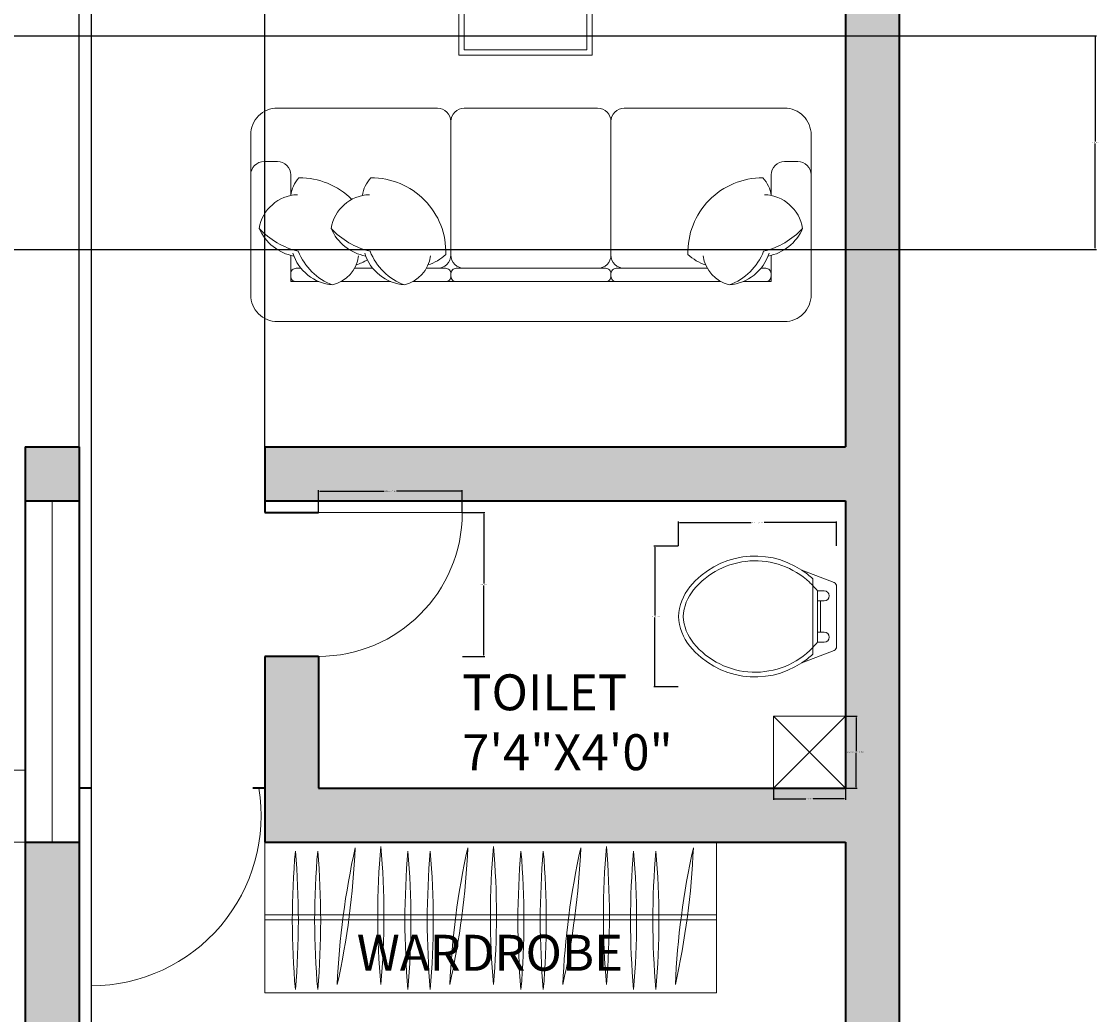
# Model space of a CAD drawing. Units: inches. Extents: x 37 to 706, y -568 to 110.
# Tile 17 of 24: x 526 to 706, y -398 to -233. Entities that reach past the tile are written whole.
import ezdxf

# ---------------------------------------------------------------- set-up
doc = ezdxf.new("R2010")
doc.units = ezdxf.units.IN
doc.header["$MEASUREMENT"] = 0
for name, color, linetype, lineweight in [('A-ANNO-DIMS', 2, 'Continuous', 18), ('A-ANNO-TEXT', 7, 'Continuous', 18), ('A-AREA-IDEN', 7, 'Continuous', 18), ('A-DOOR', 4, 'Continuous', 18), ('A-FLOR-CASE', 9, 'Continuous', 18), ('A-FLOR-FIXT', 9, 'Continuous', 18), ('A-FLOR-OPEN', 8, 'Continuous', 13), ('A-FLOR-STRS', 7, 'Continuous', 18), ('A-FURN', 8, 'Continuous', 13), ('A-GLAZ', 4, 'Continuous', 18), ('A-WALL', 7, 'Continuous', 35), ('A-WALL-PATT', 252, 'Continuous', 13)]:
    doc.layers.add(name, color=color, linetype=linetype, lineweight=lineweight)
doc.styles.get("Standard").update_dxf_attribs({"font": 'arial.ttf'})
doc.dimstyles.get("Standard").update_dxf_attribs({"dimtxt": 0.18, "dimasz": 0.18, "dimexe": 0.18, "dimexo": 0.0625, "dimgap": 0.09, "dimtad": 0, "dimtih": 1, "dimtoh": 1, "dimdec": 0, "dimzin": 0, "dimdsep": 46, "dimlunit": 3, "dimtxsty": 'Standard', "dimcen": 0.09, "dimadec": 0, "dimazin": 0, "dimtfac": 1, "dimtdec": 0, "dimtofl": 0, "dimtmove": 0, "dimatfit": 3, "dimfxl": 1, "dimtolj": 1, "dimtzin": 0, "dimarcsym": 0})

# ---------------------------------------------------------------- blocks, each defined once
blk = doc.blocks.new('WARDROBE-DOUBLE')
for p, q in [((75.49, 25.16), (0, 25.16)), ((0, 25.16), (0, 0)), ((75.49, 25.16), (75.49, 0)), ((75.49, 13), (0, 13)), ((75.49, 12.16), (0, 12.16)), ((75.49, 0), (0, 0))]:
    blk.add_line(p, q)
for centre, start, end in [((137.01, 12.08), 175.0028, 184.9972), ((-126.78, 12.08), 355.0028, 4.9972), ((140.74, 12.08), 175.0028, 184.9972), ((-123.05, 12.08), 355.0028, 4.9972), ((-117.16, 29.99), 347.508, 357.5023), ((144.38, -4.42), 167.508, 177.5023), ((151.29, 12.89), 175.0028, 184.9972), ((-112.5, 12.89), 355.0028, 4.9972), ((155.82, 12.08), 175.0028, 184.9972), ((-107.97, 12.08), 355.0028, 4.9972), ((159.55, 12.08), 175.0028, 184.9972), ((-104.24, 12.08), 355.0028, 4.9972), ((-98.35, 29.99), 347.508, 357.5023), ((163.19, -4.42), 167.508, 177.5023), ((170.1, 12.89), 175.0028, 184.9972), ((-93.69, 12.89), 355.0028, 4.9972), ((174.7, 12.08), 175.0028, 184.9972), ((-89.09, 12.08), 355.0028, 4.9972), ((178.43, 12.08), 175.0028, 184.9972), ((-85.36, 12.08), 355.0028, 4.9972), ((182.06, -4.42), 167.508, 177.5023), ((-79.47, 29.99), 347.508, 357.5023), ((188.97, 12.89), 175.0028, 184.9972), ((-74.82, 12.89), 355.0028, 4.9972), ((193.51, 12.08), 175.0028, 184.9972), ((-70.28, 12.08), 355.0028, 4.9972), ((197.24, 12.08), 175.0028, 184.9972), ((-66.55, 12.08), 355.0028, 4.9972), ((200.87, -4.42), 167.508, 177.5023), ((-60.66, 29.99), 347.508, 357.5023)]:
    blk.add_arc(centre, 132.4, start, end)
blk = doc.blocks.new('WC-PLAN')
for p, q in [((22.41, 16.39), (22.41, 15.28)), ((22.41, 15.28), (22.41, 10.09)), ((22.41, 4.89), (22.41, 10.09)), ((22.41, 4.89), (22.41, 3.79))]:
    blk.add_line(p, q)
for points in [[(20.6, 17.82, 0.383919), (1.9, 15.05, 0.163732), (0, 10.09, 0.359733)], [(21.87, 15.81, 0.431639), (2.51, 14.55, 0.162618), (0.79, 10.09, 0.470877)], [(22.41, 16.39, 0.040937), (20.6, 17.82, 0.163732)], [(26.41, 10.09), (26.41, 15.13, 0.31031), (25.98, 15.75), (20.6, 17.82, 0.209071)], [(22.41, 15.28, 0.014165), (21.87, 15.81, 0.162618)], [(23.21, 14.37, 0.022712), (22.41, 15.28, 0.162618)], [(23.21, 10.09), (23.21, 14.37, 0.022712)], [(23.21, 14.37), (24.32, 14.37, -1), (24.32, 12.69), (23.74, 12.69)], [(20.6, 2.36, -0.383919), (1.9, 5.12, -0.163732), (0, 10.09, -0.359733)], [(22.41, 4.89, -0.448546), (2.51, 5.63, -0.162618), (0.79, 10.09, -0.470877)], [(26.41, 10.09), (26.41, 5.05, -0.31031), (25.98, 4.43), (20.6, 2.36, -0.209071)], [(23.21, 10.09), (23.21, 5.8, -0.476108)], [(23.21, 5.8), (24.32, 5.8, 1), (24.32, 7.49), (23.74, 7.49)], [(23.21, 5.8, -0.022712), (22.41, 4.89, -0.162618)], [(22.41, 3.79, -0.040937), (20.6, 2.36, -0.163732)]]:
    blk.add_lwpolyline(points, format="xyb")
for points in [[(23.74, 12.69), (23.21, 12.69)], [(23.74, 7.49), (23.74, 12.69)], [(23.74, 7.49), (23.21, 7.49)]]:
    blk.add_lwpolyline(points)
blk = doc.blocks.new('COFFEE-TABLE-SQUARE')
at = {"ltscale": 0.03}
blk.add_lwpolyline([(22.29, 0), (0, 0), (0, 22.29), (22.29, 22.29)], close=True, dxfattribs=at)
blk.add_lwpolyline([(0.89, 0.89), (21.4, 0.89), (21.4, 21.4), (0.89, 21.4)], close=True)
blk = doc.blocks.new('DOOR-SWING-24')
blk.add_line((0, 0), (0, 24))
blk.add_arc((0, 0), 24, 0, 90)
blk = doc.blocks.new('FLOOR-OPENING-12-SQ')
for p, q in [((0, 0), (0, 12)), ((0, 12), (12, 12)), ((12, 12), (0, 0)), ((12, 0), (0, 12))]:
    blk.add_line(p, q)
blk = doc.blocks.new('*D17')
at = {"layer": 'A-ANNO-DIMS', "color": 0, "lineweight": -2, "transparency": 16777216}
for p, q in [((575.96, -314.65), (575.96, -310.93)), ((576.14, -311.11), (586.91, -311.11)), ((599.78, -311.11), (589, -311.11)), ((599.96, -314.65), (599.96, -310.93))]:
    blk.add_line(p, q, dxfattribs=at)
at = {"layer": 'A-ANNO-DIMS', "color": 0, "transparency": 16777216}
for points in [[(576.14, -311.08), (576.14, -311.14), (575.96, -311.11)], [(599.78, -311.08), (599.78, -311.14), (599.96, -311.11)]]:
    blk.add_solid(points, dxfattribs=at)
at = {"layer": 'Defpoints', "color": 0, "transparency": 16777216}
for p in [(599.96, -311.11), (575.96, -314.71), (599.96, -314.71)]:
    blk.add_point(p, dxfattribs=at)
at = {"layer": 'A-ANNO-DIMS', "color": 0, "transparency": 16777216, "insert": (587.96, -311.11), "char_height": 0.18, "attachment_point": 5}
blk.add_mtext('\\A1;DOOR 2\'-0" TYP.', dxfattribs=at)
blk = doc.blocks.new('*D18')
at = {"layer": 'A-ANNO-DIMS', "color": 0, "lineweight": -2, "transparency": 16777216}
for p, q in [((600.02, -314.71), (603.74, -314.71)), ((603.56, -314.89), (603.56, -326.53)), ((603.56, -338.53), (603.56, -326.89)), ((600.02, -338.71), (603.74, -338.71))]:
    blk.add_line(p, q, dxfattribs=at)
at = {"layer": 'A-ANNO-DIMS', "color": 0, "transparency": 16777216}
for points in [[(603.53, -314.89), (603.59, -314.89), (603.56, -314.71)], [(603.53, -338.53), (603.59, -338.53), (603.56, -338.71)]]:
    blk.add_solid(points, dxfattribs=at)
at = {"layer": 'Defpoints', "color": 0, "transparency": 16777216}
for p in [(599.96, -314.71), (599.96, -338.71), (603.56, -338.71)]:
    blk.add_point(p, dxfattribs=at)
at = {"layer": 'A-ANNO-DIMS', "color": 0, "transparency": 16777216, "insert": (603.56, -326.71), "char_height": 0.18, "attachment_point": 5}
blk.add_mtext('\\A1;2\'-0" TYP.', dxfattribs=at)
blk = doc.blocks.new('*D25')
at = {"layer": 'A-ANNO-DIMS', "color": 0, "lineweight": -2, "transparency": 16777216}
for p, q in [((636.09, -320.26), (636.09, -316.18)), ((636.27, -316.36), (648.2, -316.36)), ((662.32, -316.36), (650.39, -316.36)), ((662.5, -320.26), (662.5, -316.18))]:
    blk.add_line(p, q, dxfattribs=at)
at = {"layer": 'A-ANNO-DIMS', "color": 0, "transparency": 16777216}
for points in [[(636.27, -316.33), (636.27, -316.39), (636.09, -316.36)], [(662.32, -316.33), (662.32, -316.39), (662.5, -316.36)]]:
    blk.add_solid(points, dxfattribs=at)
at = {"layer": 'Defpoints', "color": 0, "transparency": 16777216}
for p in [(662.5, -316.36), (636.09, -320.32), (662.5, -320.32)]:
    blk.add_point(p, dxfattribs=at)
at = {"layer": 'A-ANNO-DIMS', "color": 0, "transparency": 16777216, "insert": (649.3, -316.36), "char_height": 0.18, "attachment_point": 5}
blk.add_mtext('\\A1;WC 2\'-2 1/2" TYP.', dxfattribs=at)
blk = doc.blocks.new('*D26')
at = {"layer": 'A-ANNO-DIMS', "color": 0, "lineweight": -2, "transparency": 16777216}
for p, q in [((636.03, -320.32), (631.95, -320.32)), ((632.13, -320.5), (632.13, -331.87)), ((632.13, -343.61), (632.13, -332.24)), ((636.03, -343.79), (631.95, -343.79))]:
    blk.add_line(p, q, dxfattribs=at)
at = {"layer": 'A-ANNO-DIMS', "color": 0, "transparency": 16777216}
for points in [[(632.1, -320.5), (632.16, -320.5), (632.13, -320.32)], [(632.1, -343.61), (632.16, -343.61), (632.13, -343.79)]]:
    blk.add_solid(points, dxfattribs=at)
at = {"layer": 'Defpoints', "color": 0, "transparency": 16777216}
for p in [(632.13, -320.32), (636.09, -320.32), (636.09, -343.79)]:
    blk.add_point(p, dxfattribs=at)
at = {"layer": 'A-ANNO-DIMS', "color": 0, "transparency": 16777216, "insert": (632.13, -332.05), "char_height": 0.18, "attachment_point": 5}
blk.add_mtext('\\A1;1\'-11 1/2" TYP.', dxfattribs=at)
blk = doc.blocks.new('*D37')
at = {"layer": 'A-ANNO-DIMS', "color": 0, "lineweight": -2, "transparency": 16777216}
for p, q in [((664.02, -348.71), (665.94, -348.71)), ((665.76, -348.89), (665.76, -354.53)), ((665.76, -360.53), (665.76, -354.89)), ((664.02, -360.71), (665.94, -360.71))]:
    blk.add_line(p, q, dxfattribs=at)
at = {"layer": 'A-ANNO-DIMS', "color": 0, "transparency": 16777216}
for points in [[(665.73, -348.89), (665.79, -348.89), (665.76, -348.71)], [(665.73, -360.53), (665.79, -360.53), (665.76, -360.71)]]:
    blk.add_solid(points, dxfattribs=at)
at = {"layer": 'Defpoints', "color": 0, "transparency": 16777216}
for p in [(663.96, -348.71), (665.76, -348.71), (663.96, -360.71)]:
    blk.add_point(p, dxfattribs=at)
at = {"layer": 'A-ANNO-DIMS', "color": 0, "transparency": 16777216, "insert": (665.76, -354.71), "char_height": 0.18, "attachment_point": 5}
blk.add_mtext('\\A1;FLOOR OPENING 1\'-0" TYP.', dxfattribs=at)
blk = doc.blocks.new('*D38')
at = {"layer": 'A-ANNO-DIMS', "color": 0, "lineweight": -2, "transparency": 16777216}
for p, q in [((651.96, -360.77), (651.96, -362.69)), ((663.96, -360.77), (663.96, -362.69)), ((652.14, -362.51), (657.33, -362.51)), ((663.78, -362.51), (658.59, -362.51))]:
    blk.add_line(p, q, dxfattribs=at)
at = {"layer": 'A-ANNO-DIMS', "color": 0, "transparency": 16777216}
for points in [[(652.14, -362.48), (652.14, -362.54), (651.96, -362.51)], [(663.78, -362.48), (663.78, -362.54), (663.96, -362.51)]]:
    blk.add_solid(points, dxfattribs=at)
at = {"layer": 'Defpoints', "color": 0, "transparency": 16777216}
for p in [(651.96, -360.71), (663.96, -360.71), (663.96, -362.51)]:
    blk.add_point(p, dxfattribs=at)
at = {"layer": 'A-ANNO-DIMS', "color": 0, "transparency": 16777216, "insert": (657.96, -362.51), "char_height": 0.18, "attachment_point": 5}
blk.add_mtext('\\A1;1\'-0" TYP.', dxfattribs=at)
blk = doc.blocks.new('*D50')
at = {"layer": 'A-ANNO-DIMS', "color": 0, "lineweight": -2, "transparency": 16777216}
for p, q in [((340.88, -235.09), (705.89, -235.09)), ((705.71, -235.27), (705.71, -252.74)), ((705.71, -270.57), (705.71, -253.1)), ((340.88, -270.75), (705.89, -270.75))]:
    blk.add_line(p, q, dxfattribs=at)
at = {"layer": 'A-ANNO-DIMS', "color": 0, "transparency": 16777216}
for points in [[(705.68, -235.27), (705.74, -235.27), (705.71, -235.09)], [(705.68, -270.57), (705.74, -270.57), (705.71, -270.75)]]:
    blk.add_solid(points, dxfattribs=at)
at = {"layer": 'Defpoints', "color": 0, "transparency": 16777216}
for p in [(340.81, -235.09), (340.81, -270.75), (705.71, -270.75)]:
    blk.add_point(p, dxfattribs=at)
at = {"layer": 'A-ANNO-DIMS', "color": 0, "transparency": 16777216, "insert": (705.71, -252.92), "char_height": 0.18, "attachment_point": 5}
blk.add_mtext('\\A1;2\'-11 1/2"', dxfattribs=at)
blk = doc.blocks.new('*D52')
at = {"layer": 'A-ANNO-DIMS', "color": 0, "lineweight": -2, "transparency": 16777216}
for p, q in [((535.96, -303.65), (535.96, 84.22)), ((536.14, 84.04), (551.13, 84.04)), ((566.78, 84.04), (551.79, 84.04)), ((566.96, -303.65), (566.96, 84.22))]:
    blk.add_line(p, q, dxfattribs=at)
at = {"layer": 'A-ANNO-DIMS', "color": 0, "transparency": 16777216}
for points in [[(536.14, 84.07), (536.14, 84.01), (535.96, 84.04)], [(566.78, 84.07), (566.78, 84.01), (566.96, 84.04)]]:
    blk.add_solid(points, dxfattribs=at)
at = {"layer": 'Defpoints', "color": 0, "transparency": 16777216}
for p in [(566.96, 84.04), (535.96, -303.71), (566.96, -303.71)]:
    blk.add_point(p, dxfattribs=at)
at = {"layer": 'A-ANNO-DIMS', "color": 0, "transparency": 16777216, "insert": (551.46, 84.04), "char_height": 0.18, "attachment_point": 5}
blk.add_mtext('\\A1;2\'-7"', dxfattribs=at)
blk = doc.blocks.new('*D53')
at = {"layer": 'A-ANNO-DIMS', "color": 0, "lineweight": -2, "transparency": 16777216}
for p, q in [((511.96, -151.77), (511.96, -567.64)), ((537.96, -151.77), (537.96, -567.64)), ((512.14, -567.46), (524.63, -567.46)), ((537.78, -567.46), (525.29, -567.46))]:
    blk.add_line(p, q, dxfattribs=at)
at = {"layer": 'A-ANNO-DIMS', "color": 0, "transparency": 16777216}
for points in [[(512.14, -567.43), (512.14, -567.49), (511.96, -567.46)], [(537.78, -567.43), (537.78, -567.49), (537.96, -567.46)]]:
    blk.add_solid(points, dxfattribs=at)
at = {"layer": 'Defpoints', "color": 0, "transparency": 16777216}
for p in [(511.96, -151.71), (537.96, -151.71), (537.96, -567.46)]:
    blk.add_point(p, dxfattribs=at)
at = {"layer": 'A-ANNO-DIMS', "color": 0, "transparency": 16777216, "insert": (524.96, -567.46), "char_height": 0.18, "attachment_point": 5}
blk.add_mtext('\\A1;2\'-2"', dxfattribs=at)

msp = doc.modelspace()

# ---------------------------------------------------------------- hatches: boundary and pattern name
at = {"layer": 'A-WALL-PATT'}
h = msp.add_hatch(color=256, dxfattribs=at)
h.dxf.hatch_style = 1
h.paths.add_polyline_path([(220.96, -351.71), (211.96, -351.71), (211.96, -513.71), (254.96, -513.71), (254.96, -504.71), (220.96, -504.71)], flags=17)
h.paths.add_polyline_path([(220.96, -294.71), (211.96, -294.71), (211.96, -303.71), (220.96, -303.71)], flags=17)
h.paths.add_polyline_path([(175.96, -294.71), (155.87, -294.71), (155.87, -303.71), (155.96, -303.71), (175.96, -303.71)], flags=17)
h.paths.add_polyline_path([(220.96, -16.71), (211.96, -16.71), (211.96, -142.71), (220.96, -142.71)], flags=17)
h.paths.add_polyline_path([(357.96, 51.29), (78.96, 51.29), (78.96, -513.71), (87.96, -513.71), (87.96, -303.71), (95.87, -303.71), (95.87, -294.71), (87.96, -294.71), (87.96, -142.71), (187.96, -142.71), (187.96, -133.71), (87.96, -133.71), (87.96, -25.71), (106.96, -25.71), (106.96, -16.71), (87.96, -16.71), (87.96, 42.29), (348.96, 42.29), (348.96, 17.13), (348.96, -133.71), (246.96, -133.71), (246.96, -142.71), (348.96, -142.71), (348.96, -294.71), (251.96, -294.71), (251.96, -303.71), (348.96, -303.71), (348.96, -351.71), (260.96, -351.71), (260.96, -329.71), (251.96, -329.71), (251.96, -360.71), (327.45, -360.71), (348.96, -360.71), (348.96, -504.71), (314.96, -504.71), (314.96, -513.71), (357.96, -513.71)])
h.paths.add_polyline_path([(416.96, -303.71), (402.96, -303.71), (402.96, -151.71), (478.96, -151.71), (478.96, -142.71), (402.96, -142.71), (402.96, -22.71), (409.96, -22.71), (409.96, -13.71), (402.96, -13.71), (402.96, 42.29), (663.96, 42.29), (663.96, -303.71), (566.96, -303.71), (566.96, -312.71), (663.96, -312.71), (663.96, -360.71), (575.96, -360.71), (575.96, -338.71), (566.96, -338.71), (566.96, -360.71), (566.96, -369.71), (642.45, -369.71), (663.96, -369.71), (663.96, -513.71), (629.96, -513.71), (629.96, -522.71), (672.96, -522.71), (672.96, 51.29), (393.96, 51.29), (393.96, -522.71), (402.96, -522.71), (402.96, -312.71), (416.96, -312.71)])
h.paths.add_polyline_path([(490.96, -303.71), (476.96, -303.71), (476.96, -312.71), (490.96, -312.71)], flags=17)
h.paths.add_polyline_path([(535.96, -303.71), (526.96, -303.71), (526.96, -312.71), (535.96, -312.71)], flags=17)
h.paths.add_polyline_path([(535.96, -369.71), (526.96, -369.71), (526.96, -522.71), (569.96, -522.71), (569.96, -513.71), (535.96, -513.71)], flags=17)
h.paths.add_polyline_path([(511.96, -13.71), (502.96, -13.71), (502.96, -151.71), (511.96, -151.71)], flags=17)
h.paths.add_polyline_path([(651.54, -142.71), (651.54, -120.18), (642.54, -120.18), (642.54, -142.71), (550.54, -142.71), (550.54, -120.71), (541.54, -120.71), (541.54, -142.71), (537.96, -142.71), (537.96, -151.71), (651.54, -151.71)], flags=17)
h.paths.add_polyline_path([(651.54, -85.71), (541.54, -85.71), (541.54, -94.71), (651.54, -94.71)], flags=17)
h.paths.add_polyline_path([(476.96, -13.71), (469.96, -13.71), (469.96, -22.71), (476.96, -22.71)], flags=17)
h.paths.add_polyline_path([(185.96, -16.71), (166.96, -16.71), (166.96, -25.71), (185.96, -25.71)], flags=17)
h.paths.add_polyline_path([(168.91, -414.72), (214.62, -414.72), (214.62, -392.33), (168.91, -392.33)], flags=25)

# ---------------------------------------------------------------- linework, layer by layer
at = {"layer": 'A-DOOR'}
msp.add_line((537.96, -360.71), (537.96, -393.71), dxfattribs=at)
msp.add_arc((537.96, -365.33), 28.38, 270, 9.3718, dxfattribs=at)
at = {"layer": 'A-FLOR-STRS'}
for p, q in [((490.96, -357.71), (526.96, -357.71)), ((490.96, -369.71), (526.96, -369.71))]:
    msp.add_line(p, q, dxfattribs=at)
at = {"layer": 'A-FURN', "ltscale": 0.03}
msp.add_lwpolyline([(658.24, -251.62, 0.414214), (653.78, -247.16), (627.03, -247.16, 0.414214), (624.8, -249.39, 0.414214), (622.57, -247.16), (600.29, -247.16, 0.414214), (598.06, -249.39, 0.414214), (595.83, -247.16), (569.08, -247.16, 0.414214), (564.62, -251.62), (564.62, -278.36, 0.414214), (569.08, -282.82), (653.78, -282.82, 0.414214), (658.24, -278.36)], format="xyb", close=True, dxfattribs=at)
at = {"layer": 'A-FURN'}
for points in [[(595.83, -273.91, 0.414214), (598.06, -271.68), (598.06, -249.39, 0.414214)], [(627.03, -273.91, -0.414214), (624.8, -271.68), (624.8, -249.39, -0.414214)], [(571.31, -261.76), (571.31, -258.3, 0.414214), (569.08, -256.07), (566.85, -256.07, 0.414214), (564.62, -258.3)], [(658.24, -258.3, 0.414214), (656.01, -256.07), (653.78, -256.07, 0.414214), (651.55, -258.3), (651.55, -261.76)], [(571.31, -261.76, -0.165541), (572.68, -258.81, -0.200231), (581.53, -262.4, -0.121523)], [(583.31, -261.76, -0.165541), (584.69, -258.81, -0.425989), (597.21, -271.58, -0.121523), (594.24, -273.34, 7.115464)], [(651.55, -261.76, 0.165541), (650.18, -258.81, 0.425989), (637.66, -271.58, 0.121523), (640.63, -273.34, -7.115464)], [(572.43, -261.62, 0.356772), (566.04, -267.24, 0.249542), (571.83, -271.87, -9.61688)], [(584.44, -261.62, 0.356772), (578.05, -267.24, 0.249542), (583.84, -271.87, -9.61688)], [(650.43, -261.62, -0.356772), (656.82, -267.24, -0.249542), (651.03, -271.87, 9.61688)], [(566.04, -267.24, 0.14773), (572.56, -271.07, 0.213343), (578.3, -276.69, 0.178662)], [(578.05, -267.24, 0.14773), (584.56, -271.07, 0.213343), (590.31, -276.69, 0.178662)], [(656.82, -267.24, -0.14773), (650.3, -271.07, -0.213343), (644.56, -276.69, -0.178662)], [(571.66, -271.38, 0.306663), (578.3, -276.69, 0.30633), (582.65, -271.84, -0.872847)], [(583.66, -271.38, 0.306663), (590.31, -276.69, 0.30633), (594.65, -271.84, -0.872847)], [(651.2, -271.38, -0.306663), (644.56, -276.69, -0.30633), (640.21, -271.84, 0.872847)], [(576, -276.13), (571.31, -276.13), (571.31, -271.75, 0.414214)], [(584.1, -272.47, -0.071865), (582.23, -273.34, 7.115464)], [(600.29, -273.91, -0.414214), (598.06, -271.68)], [(622.57, -273.91, 0.414214), (624.8, -271.68)], [(573.01, -273.91), (572.2, -273.91, 0.414214), (571.31, -274.8), (571.31, -275.24, 0.414214), (572.2, -276.13)], [(585.02, -273.91), (581.95, -273.91, 0.414214)], [(591.71, -276.13), (597.17, -276.13, 0.414214), (598.06, -275.24), (598.06, -274.8, 0.414214), (597.17, -273.91), (593.96, -273.91, 0.414214)], [(643.15, -276.13), (625.69, -276.13, -0.414214), (624.8, -275.24), (624.8, -274.8, -0.414214), (625.69, -273.91), (640.91, -273.91, -0.414214)], [(649.85, -273.91), (650.66, -273.91, -0.414214), (651.55, -274.8), (651.55, -275.24, -0.414214), (650.66, -276.13)], [(572.2, -276.13), (576, -276.13, 0.414214)], [(579.71, -276.13), (588.01, -276.13, 0.414214)], [(650.66, -276.13), (646.86, -276.13, -0.414214)]]:
    msp.add_lwpolyline(points, format="xyb", dxfattribs=at)
for points in [[(651.55, -271.75), (651.55, -276.13), (646.86, -276.13)], [(588.01, -276.13), (579.71, -276.13)], [(643.15, -276.13), (591.71, -276.13)]]:
    msp.add_lwpolyline(points, dxfattribs=at)
msp.add_lwpolyline([(598.95, -276.13), (623.91, -276.13, 0.414214), (624.8, -275.24), (624.8, -274.8, 0.414214), (623.91, -273.91), (598.95, -273.91, 0.414214), (598.06, -274.8), (598.06, -275.24, 0.414214)], format="xyb", close=True, dxfattribs=at)
at = {"layer": 'A-GLAZ'}
msp.add_line((531.46, -369.71), (531.46, -312.71), dxfattribs=at)
at = {"layer": 'A-WALL'}
for p, q in [((672.96, 51.29), (672.96, -522.71)), ((663.96, 42.29), (663.96, -303.71)), ((526.96, -303.71), (526.96, -522.71)), ((526.96, -303.71), (535.96, -303.71)), ((535.96, -303.71), (535.96, -513.71)), ((566.96, -303.71), (566.96, -314.71)), ((566.96, -303.71), (663.96, -303.71)), ((526.96, -312.71), (535.96, -312.71)), ((566.96, -312.71), (663.96, -312.71)), ((663.96, -312.71), (663.96, -360.71)), ((566.96, -314.71), (575.96, -314.71)), ((575.96, -338.71), (566.96, -338.71)), ((566.96, -338.71), (566.96, -360.71)), ((575.96, -338.71), (575.96, -360.71)), ((537.96, -360.71), (535.96, -360.71)), ((566.96, -360.71), (564.96, -360.71)), ((566.96, -360.71), (566.96, -369.71)), ((575.96, -360.71), (663.96, -360.71)), ((526.96, -369.71), (535.96, -369.71)), ((566.96, -369.71), (663.96, -369.71)), ((663.96, -369.71), (663.96, -513.71))]:
    msp.add_line(p, q, dxfattribs=at)

# ---------------------------------------------------------------- block references
at = {"layer": 'A-DOOR', "rotation": 269.9999999999999}
msp.add_blockref('DOOR-SWING-24', (575.96, -314.71), dxfattribs=at)
at = {"layer": 'A-FLOR-CASE'}
msp.add_blockref('WARDROBE-DOUBLE', (566.96, -394.87), dxfattribs=at)
at = {"layer": 'A-FLOR-FIXT'}
msp.add_blockref('WC-PLAN', (636.09, -342.14), dxfattribs=at)
at = {"layer": 'A-FLOR-OPEN'}
msp.add_blockref('FLOOR-OPENING-12-SQ', (651.96, -360.71), dxfattribs=at)
at = {"layer": 'A-FURN'}
msp.add_blockref('COFFEE-TABLE-SQUARE', (599.38, -238.33), dxfattribs=at)

# ---------------------------------------------------------------- texts
at = {"layer": 'A-ANNO-TEXT', "insert": (582.34, -385.2), "char_height": 6, "attachment_point": 1}
msp.add_mtext_dynamic_manual_height_columns('WARDROBE', width=0.234, gutter_width=1, heights=[0], dxfattribs=at)
at = {"layer": 'A-AREA-IDEN', "insert": (599.95, -341.71), "char_height": 6, "attachment_point": 1}
msp.add_mtext('TOILET\\P7\'4"X4\'0"', dxfattribs=at)

# ---------------------------------------------------------------- dimensions: what is measured, and where the dimension line sits
at = {"layer": 'A-ANNO-DIMS'}
for base, p1, p2, picture, middle in [((566.96, 84.04), (535.96, -303.71), (566.96, -303.71), '*D52', (551.46, 84.04)), ((537.96, -567.46), (511.96, -151.71), (537.96, -151.71), '*D53', (524.96, -567.46))]:
    dim = msp.add_linear_dim(base=base, p1=p1, p2=p2, dimstyle='Standard', override={"dimdec": 1, "dimlfac": 1, "dimrnd": 0, "dimzin": 1, "dimdsep": 46, "dimlunit": 4, "dimfrac": 2}, dxfattribs=at)
    dim.commit()
    dim.dimension.update_dxf_attribs({"geometry": picture, "text_midpoint": middle})
dim = msp.add_linear_dim(base=(705.71, -270.75), p1=(340.81, -235.09), p2=(340.81, -270.75), angle=90, dimstyle='Standard', override={"dimdec": 1, "dimlfac": 1, "dimrnd": 0, "dimzin": 1, "dimdsep": 46, "dimlunit": 4, "dimfrac": 2}, dxfattribs=at)
dim.commit()
dim.dimension.update_dxf_attribs({"geometry": '*D50', "text_midpoint": (705.71, -252.92)})
for base, p1, p2, text, picture, middle in [((599.96, -311.11), (575.96, -314.71), (599.96, -314.71), 'DOOR <> TYP.', '*D17', (587.96, -311.11)), ((662.5, -316.36), (636.09, -320.32), (662.5, -320.32), 'WC <> TYP.', '*D25', (649.3, -316.36)), ((663.96, -362.51), (651.96, -360.71), (663.96, -360.71), '<> TYP.', '*D38', (657.96, -362.51))]:
    dim = msp.add_linear_dim(base=base, p1=p1, p2=p2, text=text, dimstyle='Standard', override={"dimdec": 1, "dimlfac": 1, "dimrnd": 0, "dimzin": 1, "dimdsep": 46, "dimlunit": 4, "dimfrac": 2}, dxfattribs=at)
    dim.commit()
    dim.dimension.update_dxf_attribs({"geometry": picture, "text_midpoint": middle})
for base, p1, p2, angle, text, picture, middle in [((603.56, -338.71), (599.96, -314.71), (599.96, -338.71), 270, '<> TYP.', '*D18', (603.56, -326.71)), ((632.13, -320.32), (636.09, -343.79), (636.09, -320.32), 90, '<> TYP.', '*D26', (632.13, -332.05)), ((665.76, -348.71), (663.96, -360.71), (663.96, -348.71), 90, 'FLOOR OPENING <> TYP.', '*D37', (665.76, -354.71))]:
    dim = msp.add_linear_dim(base=base, p1=p1, p2=p2, angle=angle, text=text, dimstyle='Standard', override={"dimdec": 1, "dimlfac": 1, "dimrnd": 0, "dimzin": 1, "dimdsep": 46, "dimlunit": 4, "dimfrac": 2}, dxfattribs=at)
    dim.commit()
    dim.dimension.update_dxf_attribs({"geometry": picture, "text_midpoint": middle})

doc.saveas('drawing.dxf')
